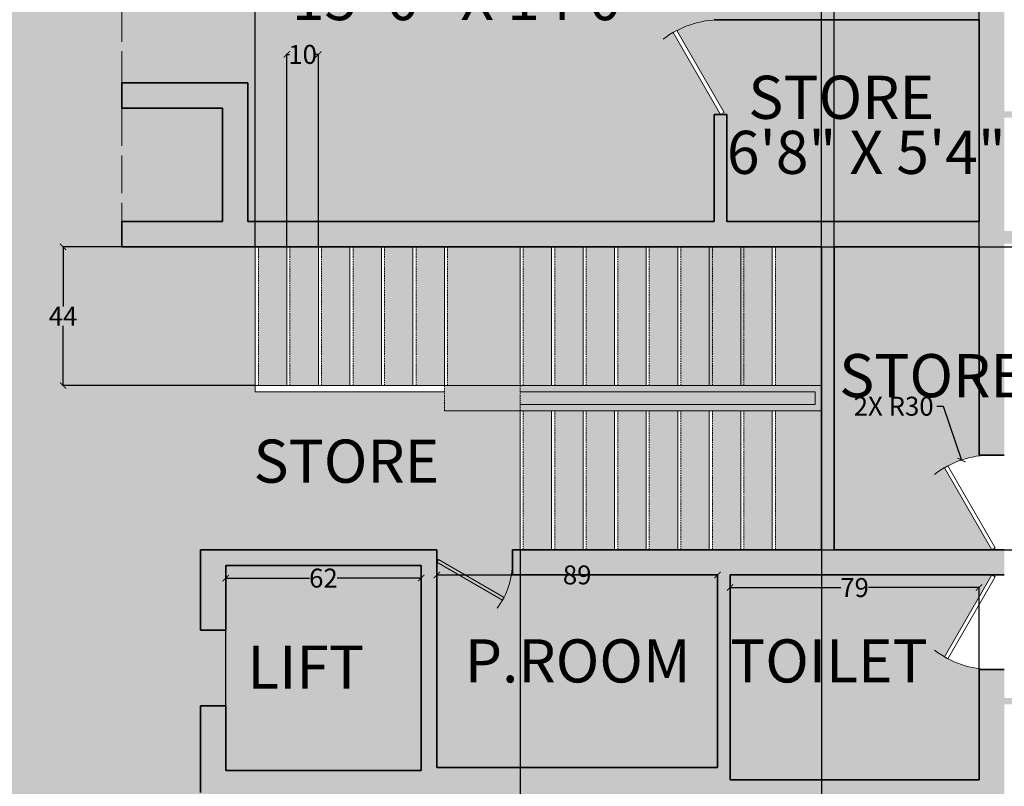
# Model space of a CAD drawing. Units: inches. Extents: x 1704 to 6393, y -157 to 1172.
# Tile 87 of 122: x 2293 to 2605, y 540 to 783. Entities that reach past the tile are written whole.
import ezdxf

# ---------------------------------------------------------------- set-up
doc = ezdxf.new("R2010")
doc.units = ezdxf.units.IN
doc.header["$MEASUREMENT"] = 0
doc.linetypes.add('ACAD_ISO02W100', pattern=[15, 12, -3])
doc.linetypes.add('DASHED', pattern=[0.75, 0.5, -0.25])
for name, color, linetype, lineweight in [('A-ANNO-DIMS', 7, 'Continuous', 13), ('A-AREA-IDEN', 7, 'Continuous', 18), ('A-FLOR-STRS-HIDN', 8, 'DASHED', 13), ('A-WALL-OVHD', 8, 'ACAD_ISO02W100', 13), ('A-WALL-PATT', 7, 'Continuous', 13), ('DOORS', 160, 'Continuous', 18), ('STAIRS', 7, 'Continuous', 18), ('WALLS', 7, 'Continuous', 35)]:
    doc.layers.add(name, color=color, linetype=linetype, lineweight=lineweight)
doc.layers.add('A-FLOR-PATT', color=7, linetype='Continuous', lineweight=13, true_color=0xf2f2f2)
doc.styles.get("Standard").update_dxf_attribs({"font": 'arial.ttf'})
doc.dimstyles.get("Standard").update_dxf_attribs({"dimtxt": 6, "dimasz": 2, "dimexe": 0.18, "dimexo": 0.0625, "dimgap": 0.09, "dimtad": 0, "dimtih": 1, "dimtoh": 1, "dimdec": 1, "dimzin": 0, "dimdsep": 46, "dimlunit": 3, "dimtxsty": 'Standard', "dimblk": 'ARCHTICK', "dimcen": 0.09, "dimadec": 0, "dimazin": 0, "dimtfac": 1, "dimtdec": 1, "dimtofl": 0, "dimtmove": 0, "dimatfit": 3, "dimfxl": 1, "dimtolj": 1, "dimtzin": 0, "dimarcsym": 0})

# ---------------------------------------------------------------- blocks, each defined once
blk = doc.blocks.new('Door - Left Hung 36 in.')
blk.add_lwpolyline([(0.75, -1.3), (0, 0), (31.18, 18), (31.93, 16.7)], close=True)
blk.add_arc((0, 0), 36, 0, 37.3101)
blk = doc.blocks.new('_ArchTick')
at = {"color": 0, "linetype": 'ByBlock', "const_width": 0.15}
blk.add_lwpolyline([(-0.5, -0.5), (0.5, 0.5)], dxfattribs=at)
blk = doc.blocks.new('*D93')
at = {"layer": 'A-ANNO-DIMS', "color": 0, "lineweight": -2, "transparency": 16777216}
for p, q in [((2605.29, 895.21), (1829.7, 895.21)), ((1829.88, 895.21), (1829.88, 495.87)), ((1829.88, 90.21), (1829.88, 489.56)), ((2605.29, 90.21), (1829.7, 90.21))]:
    blk.add_line(p, q, dxfattribs=at)
at = {"layer": 'Defpoints', "color": 0, "lineweight": -3, "transparency": 16777216}
for p in [(2605.35, 895.21), (1829.88, 90.21), (2605.35, 90.21)]:
    blk.add_point(p, dxfattribs=at)
at = {"layer": 'A-ANNO-DIMS', "color": 0, "lineweight": -2, "transparency": 16777216, "xscale": 2, "yscale": 2, "zscale": 2}
for p, rotation in [((1829.88, 895.21), 90), ((1829.88, 90.21), 270)]:
    blk.add_blockref('_ArchTick', p, dxfattribs=dict(at, rotation=rotation))
at = {"layer": 'A-ANNO-DIMS', "color": 0, "transparency": 16777216, "insert": (1829.88, 492.71), "char_height": 6, "attachment_point": 5}
blk.add_mtext('\\A1;805', dxfattribs=at)
blk = doc.blocks.new('*D98')
at = {"layer": 'A-ANNO-DIMS', "color": 0, "lineweight": -2, "transparency": 16777216}
for p, q in [((2358.35, 545.28), (2358.35, 606.39)), ((2358.35, 606.21), (2384.98, 606.21)), ((2420.35, 606.21), (2393.72, 606.21)), ((2420.35, 545.28), (2420.35, 606.39))]:
    blk.add_line(p, q, dxfattribs=at)
at = {"layer": 'Defpoints', "color": 0, "lineweight": -3, "transparency": 16777216}
for p in [(2420.35, 606.21), (2358.35, 545.21), (2420.35, 545.21)]:
    blk.add_point(p, dxfattribs=at)
at = {"layer": 'A-ANNO-DIMS', "color": 0, "lineweight": -2, "transparency": 16777216, "xscale": 2, "yscale": 2, "zscale": 2, "rotation": 180}
blk.add_blockref('_ArchTick', (2358.35, 606.21), dxfattribs=at)
at = {"layer": 'A-ANNO-DIMS', "color": 0, "lineweight": -2, "transparency": 16777216, "xscale": 2, "yscale": 2, "zscale": 2}
blk.add_blockref('_ArchTick', (2420.35, 606.21), dxfattribs=at)
at = {"layer": 'A-ANNO-DIMS', "color": 0, "transparency": 16777216, "insert": (2389.35, 606.21), "char_height": 6, "attachment_point": 5}
blk.add_mtext('\\A1;62', dxfattribs=at)
blk = doc.blocks.new('*D99')
at = {"layer": 'A-ANNO-DIMS', "color": 0, "lineweight": -2, "transparency": 16777216}
for p, q in [((2425.35, 546.28), (2425.35, 607.39)), ((2425.35, 607.21), (2465.45, 607.21)), ((2514.35, 607.21), (2474.25, 607.21)), ((2514.35, 546.28), (2514.35, 607.39))]:
    blk.add_line(p, q, dxfattribs=at)
at = {"layer": 'Defpoints', "color": 0, "lineweight": -3, "transparency": 16777216}
for p in [(2514.35, 607.21), (2425.35, 546.21), (2514.35, 546.21)]:
    blk.add_point(p, dxfattribs=at)
at = {"layer": 'A-ANNO-DIMS', "color": 0, "lineweight": -2, "transparency": 16777216, "xscale": 2, "yscale": 2, "zscale": 2, "rotation": 180}
blk.add_blockref('_ArchTick', (2425.35, 607.21), dxfattribs=at)
at = {"layer": 'A-ANNO-DIMS', "color": 0, "lineweight": -2, "transparency": 16777216, "xscale": 2, "yscale": 2, "zscale": 2}
blk.add_blockref('_ArchTick', (2514.35, 607.21), dxfattribs=at)
at = {"layer": 'A-ANNO-DIMS', "color": 0, "transparency": 16777216, "insert": (2469.85, 607.21), "char_height": 6, "attachment_point": 5}
blk.add_mtext('\\A1;89', dxfattribs=at)
blk = doc.blocks.new('*D100')
at = {"layer": 'A-ANNO-DIMS', "color": 0, "lineweight": -2, "transparency": 16777216}
for p, q in [((2518.35, 542.28), (2518.35, 603.39)), ((2518.35, 603.21), (2553.48, 603.21)), ((2597.35, 603.21), (2562.22, 603.21)), ((2597.35, 542.28), (2597.35, 603.39))]:
    blk.add_line(p, q, dxfattribs=at)
at = {"layer": 'Defpoints', "color": 0, "lineweight": -3, "transparency": 16777216}
for p in [(2597.35, 603.21), (2518.35, 542.21), (2597.35, 542.21)]:
    blk.add_point(p, dxfattribs=at)
at = {"layer": 'A-ANNO-DIMS', "color": 0, "lineweight": -2, "transparency": 16777216, "xscale": 2, "yscale": 2, "zscale": 2, "rotation": 180}
blk.add_blockref('_ArchTick', (2518.35, 603.21), dxfattribs=at)
at = {"layer": 'A-ANNO-DIMS', "color": 0, "lineweight": -2, "transparency": 16777216, "xscale": 2, "yscale": 2, "zscale": 2}
blk.add_blockref('_ArchTick', (2597.35, 603.21), dxfattribs=at)
at = {"layer": 'A-ANNO-DIMS', "color": 0, "transparency": 16777216, "insert": (2557.85, 603.21), "char_height": 6, "attachment_point": 5}
blk.add_mtext('\\A1;79', dxfattribs=at)
blk = doc.blocks.new('*D101')
at = {"layer": 'A-ANNO-DIMS', "color": 0, "lineweight": -2, "transparency": 16777216}
for p, q in [((2547.41, 711.21), (2784.53, 711.21)), ((2784.35, 711.21), (2784.35, 666.37)), ((2784.35, 615.21), (2784.35, 660.06)), ((2547.41, 615.21), (2784.53, 615.21))]:
    blk.add_line(p, q, dxfattribs=at)
at = {"layer": 'Defpoints', "color": 0, "lineweight": -3, "transparency": 16777216}
for p in [(2547.35, 711.21), (2784.35, 711.21), (2547.35, 615.21)]:
    blk.add_point(p, dxfattribs=at)
at = {"layer": 'A-ANNO-DIMS', "color": 0, "lineweight": -2, "transparency": 16777216, "xscale": 2, "yscale": 2, "zscale": 2}
for p, rotation in [((2784.35, 711.21), 90), ((2784.35, 615.21), 270)]:
    blk.add_blockref('_ArchTick', p, dxfattribs=dict(at, rotation=rotation))
at = {"layer": 'A-ANNO-DIMS', "color": 0, "transparency": 16777216, "insert": (2784.35, 663.21), "char_height": 6, "attachment_point": 5}
blk.add_mtext('\\A1;96', dxfattribs=at)
blk = doc.blocks.new('*D102')
at = {"layer": 'A-ANNO-DIMS', "color": 0, "lineweight": -2, "transparency": 16777216}
for p, q in [((2367.74, 711.28), (2367.74, 1105.29)), ((2367.74, 1105.11), (2447.61, 1105.11)), ((2547.35, 1105.11), (2467.47, 1105.11)), ((2547.35, 711.28), (2547.35, 1105.29))]:
    blk.add_line(p, q, dxfattribs=at)
at = {"layer": 'Defpoints', "color": 0, "lineweight": -3, "transparency": 16777216}
for p in [(2547.35, 1105.11), (2367.74, 711.21), (2547.35, 711.21)]:
    blk.add_point(p, dxfattribs=at)
at = {"layer": 'A-ANNO-DIMS', "color": 0, "lineweight": -2, "transparency": 16777216, "xscale": 2, "yscale": 2, "zscale": 2, "rotation": 180}
blk.add_blockref('_ArchTick', (2367.74, 1105.11), dxfattribs=at)
at = {"layer": 'A-ANNO-DIMS', "color": 0, "lineweight": -2, "transparency": 16777216, "xscale": 2, "yscale": 2, "zscale": 2}
blk.add_blockref('_ArchTick', (2547.35, 1105.11), dxfattribs=at)
at = {"layer": 'A-ANNO-DIMS', "color": 0, "transparency": 16777216, "insert": (2457.54, 1105.11), "char_height": 6, "attachment_point": 5}
blk.add_mtext('\\A1;179.6', dxfattribs=at)
blk = doc.blocks.new('*D103')
at = {"layer": 'A-ANNO-DIMS', "color": 0, "lineweight": -2, "transparency": 16777216}
for p, q in [((2551.35, 711.28), (2551.35, 1105.29)), ((2551.35, 1105.11), (2569.84, 1105.11)), ((2597.35, 1105.11), (2578.85, 1105.11)), ((2597.35, 711.28), (2597.35, 1105.29))]:
    blk.add_line(p, q, dxfattribs=at)
at = {"layer": 'Defpoints', "color": 0, "lineweight": -3, "transparency": 16777216}
for p in [(2597.35, 1105.11), (2551.35, 711.21), (2597.35, 711.21)]:
    blk.add_point(p, dxfattribs=at)
at = {"layer": 'A-ANNO-DIMS', "color": 0, "lineweight": -2, "transparency": 16777216, "xscale": 2, "yscale": 2, "zscale": 2, "rotation": 180}
blk.add_blockref('_ArchTick', (2551.35, 1105.11), dxfattribs=at)
at = {"layer": 'A-ANNO-DIMS', "color": 0, "lineweight": -2, "transparency": 16777216, "xscale": 2, "yscale": 2, "zscale": 2}
blk.add_blockref('_ArchTick', (2597.35, 1105.11), dxfattribs=at)
at = {"layer": 'A-ANNO-DIMS', "color": 0, "transparency": 16777216, "insert": (2574.35, 1105.11), "char_height": 6, "attachment_point": 5}
blk.add_mtext('\\A1;46', dxfattribs=at)
blk = doc.blocks.new('*D104')
at = {"layer": 'A-ANNO-DIMS', "color": 0, "lineweight": -2, "transparency": 16777216}
for p, q in [((2367.675475, 711.212974), (2306.557975, 711.212974)), ((2306.737975, 711.212974), (2306.737975, 692.302974)), ((2306.737975, 667.212974), (2306.737975, 686.122974)), ((2367.675475, 667.212974), (2306.557975, 667.212974))]:
    blk.add_line(p, q, dxfattribs=at)
at = {"layer": 'Defpoints', "color": 0, "lineweight": -3, "transparency": 16777216}
for p in [(2306.737975, 711.212974), (2367.737975, 711.212974), (2367.737975, 667.212974)]:
    blk.add_point(p, dxfattribs=at)
at = {"layer": 'A-ANNO-DIMS', "color": 0, "lineweight": -2, "transparency": 16777216, "xscale": 2, "yscale": 2, "zscale": 2}
for p, rotation in [((2306.737975, 711.212974), 90), ((2306.737975, 667.212974), 270)]:
    blk.add_blockref('_ArchTick', p, dxfattribs=dict(at, rotation=rotation))
at = {"layer": 'A-ANNO-DIMS', "color": 0, "transparency": 16777216, "insert": (2306.737975, 689.212974), "char_height": 6, "attachment_point": 5}
blk.add_mtext('\\A1;44', dxfattribs=at)
blk = doc.blocks.new('*D105')
at = {"layer": 'A-ANNO-DIMS', "color": 0, "lineweight": -2, "transparency": 16777216}
for p, q in [((2451.74, 615.15), (2451.74, -64.97)), ((2547.35, 615.15), (2547.35, -64.97)), ((2451.74, -64.79), (2489.91, -64.79)), ((2547.35, -64.79), (2509.18, -64.79))]:
    blk.add_line(p, q, dxfattribs=at)
at = {"layer": 'Defpoints', "color": 0, "lineweight": -3, "transparency": 16777216}
for p in [(2451.74, 615.21), (2547.35, 615.21), (2547.35, -64.79)]:
    blk.add_point(p, dxfattribs=at)
at = {"layer": 'A-ANNO-DIMS', "color": 0, "lineweight": -2, "transparency": 16777216, "xscale": 2, "yscale": 2, "zscale": 2, "rotation": 180}
blk.add_blockref('_ArchTick', (2451.74, -64.79), dxfattribs=at)
at = {"layer": 'A-ANNO-DIMS', "color": 0, "lineweight": -2, "transparency": 16777216, "xscale": 2, "yscale": 2, "zscale": 2}
blk.add_blockref('_ArchTick', (2547.35, -64.79), dxfattribs=at)
at = {"layer": 'A-ANNO-DIMS', "color": 0, "transparency": 16777216, "insert": (2499.54, -64.79), "char_height": 6, "attachment_point": 5}
blk.add_mtext('\\A1;95.61', dxfattribs=at)
blk = doc.blocks.new('*D106')
at = {"layer": 'A-ANNO-DIMS', "color": 0, "lineweight": -2, "transparency": 16777216}
for p, q in [((2377.74, 711.28), (2377.74, 772.39)), ((2377.74, 772.21), (2378.64, 772.21)), ((2387.74, 772.21), (2386.83, 772.21)), ((2387.74, 711.28), (2387.74, 772.39))]:
    blk.add_line(p, q, dxfattribs=at)
at = {"layer": 'Defpoints', "color": 0, "lineweight": -3, "transparency": 16777216}
for p in [(2387.74, 772.21), (2377.74, 711.21), (2387.74, 711.21)]:
    blk.add_point(p, dxfattribs=at)
at = {"layer": 'A-ANNO-DIMS', "color": 0, "lineweight": -2, "transparency": 16777216, "xscale": 2, "yscale": 2, "zscale": 2, "rotation": 180}
blk.add_blockref('_ArchTick', (2377.74, 772.21), dxfattribs=at)
at = {"layer": 'A-ANNO-DIMS', "color": 0, "lineweight": -2, "transparency": 16777216, "xscale": 2, "yscale": 2, "zscale": 2}
blk.add_blockref('_ArchTick', (2387.74, 772.21), dxfattribs=at)
at = {"layer": 'A-ANNO-DIMS', "color": 0, "transparency": 16777216, "insert": (2382.74, 772.21), "char_height": 6, "attachment_point": 5}
blk.add_mtext('\\A1;10', dxfattribs=at)
blk = doc.blocks.new('*D136')
at = {"layer": 'A-ANNO-DIMS', "color": 0, "lineweight": -2, "transparency": 16777216}
for p, q in [((2583.99, 660.69), (2585.99, 660.69)), ((2585.99, 660.69), (2591.75, 643.64)), ((2601.26, 615.21), (2601.44, 615.21)), ((2601.35, 615.12), (2601.35, 615.3))]:
    blk.add_line(p, q, dxfattribs=at)
at = {"layer": 'Defpoints', "color": 0, "lineweight": -3, "transparency": 16777216}
for p in [(2591.75, 643.64), (2601.35, 615.21)]:
    blk.add_point(p, dxfattribs=at)
at = {"layer": 'A-ANNO-DIMS', "color": 0, "lineweight": -2, "transparency": 16777216, "xscale": 2, "yscale": 2, "zscale": 2, "rotation": 288.6558092549602}
blk.add_blockref('_ArchTick', (2591.75, 643.64), dxfattribs=at)
at = {"layer": 'A-ANNO-DIMS', "color": 0, "transparency": 16777216, "insert": (2570.25, 660.69), "char_height": 6, "attachment_point": 5}
blk.add_mtext('\\A1;2X R30', dxfattribs=at)

msp = doc.modelspace()

# ---------------------------------------------------------------- hatches: boundary and pattern name
at = {"layer": 'A-FLOR-PATT', "transparency": 33554528}
h = msp.add_hatch(color=256, dxfattribs=at)
h.dxf.hatch_style = 1
h.paths.add_polyline_path([(2325.349, 863.213), (2325.349, 887.213), (2263.349, 887.213), (2167.349, 887.213), (2081.349, 887.213), (2081.349, 719.213), (2277.349, 719.213), (2277.349, 711.213), (2277.349, 372.213), (2349.349, 372.213), (2381.349, 372.213), (2381.349, 364.213), (2353.349, 364.213), (2353.349, 270.213), (2381.349, 270.213), (2381.349, 266.213), (2357.349, 266.213), (2357.349, 98.213), (2381.349, 98.213), (2385.181, 98.213), (2386.482, 98.213), (2424.215, 98.213), (2425.516, 98.213), (2429.349, 98.213), (2597.349, 98.213), (2597.349, 146.213), (2597.349, 218.213), (2597.349, 266.213), (2423.349, 266.213), (2423.349, 270.213), (2473.349, 270.213), (2473.349, 294.213), (2477.349, 294.213), (2477.349, 270.213), (2547.349, 270.213), (2547.349, 364.213), (2477.349, 364.213), (2477.349, 318.213), (2473.349, 318.213), (2473.349, 364.213), (2423.349, 364.213), (2423.349, 372.213), (2469.349, 372.213), (2469.349, 459.213), (2469.349, 538.213), (2350.349, 538.213), (2350.349, 565.713), (2358.349, 565.713), (2358.349, 545.213), (2420.349, 545.213), (2420.349, 610.213), (2358.349, 610.213), (2358.349, 589.713), (2350.349, 589.713), (2350.349, 615.213), (2425.349, 615.213), (2425.349, 607.213), (2425.349, 546.213), (2469.349, 546.213), (2514.349, 546.213), (2514.349, 607.213), (2449.349, 607.213), (2449.349, 615.213), (2451.738, 615.213), (2451.738, 659.213), (2427.738, 659.213), (2427.738, 665.213), (2367.738, 665.213), (2367.738, 667.213), (2367.738, 711.213), (2325.349, 711.213), (2325.349, 719.213), (2325.349, 755.213), (2325.349, 763.213)])
h.paths.add_polyline_path([(2233.858, 822.533, -0.187247), (2233.858, 809.14), (2231.697, 808.804, 0.0848928), (2233.131, 814.486), (2230.424, 814.486, -0.1042581), (2228.553, 808.313), (2217.751, 807.156, -0.2222222), (2217.751, 824.517), (2228.553, 823.359, -0.1042581), (2230.424, 817.186), (2233.131, 817.186, 0.0848928), (2231.697, 822.868)], flags=16)
h.paths.add_polyline_path([(2213.621, 833.197), (2213.621, 798.475), (2156.048, 798.475), (2156.048, 833.197)], flags=16)
h.paths.add_polyline_path([(2203.932, 848.099), (2205.089, 837.296, -0.2222222), (2187.728, 837.296), (2188.885, 848.099, -0.1042581), (2195.058, 849.969), (2195.058, 852.676, 0.0848928), (2189.377, 851.242), (2189.712, 853.404, -0.187247), (2203.105, 853.404), (2203.44, 851.242, 0.0848928), (2197.759, 852.676), (2197.759, 849.969, -0.1042581)], flags=16)
h.paths.add_polyline_path([(2181.941, 837.296, -0.2222222), (2164.58, 837.296), (2165.737, 848.099, -0.1042581), (2171.91, 849.969), (2171.91, 852.676, 0.0848928), (2166.229, 851.242), (2166.564, 853.404, -0.187247), (2179.957, 853.404), (2180.292, 851.242, 0.0848928), (2174.611, 852.676), (2174.611, 849.969, -0.1042581), (2180.784, 848.099)], flags=16)
h.paths.add_polyline_path([(2205.089, 794.376), (2203.932, 783.574, -0.1042581), (2197.759, 781.703), (2197.759, 778.996, 0.0848928), (2203.44, 780.43), (2203.105, 778.269, -0.187247), (2189.712, 778.269), (2189.377, 780.43, 0.0848928), (2195.058, 778.996), (2195.058, 781.703, -0.1042581), (2188.885, 783.574), (2187.728, 794.376, -0.2222222)], flags=16)
h.paths.add_polyline_path([(2181.941, 794.376), (2180.784, 783.574, -0.1042581), (2174.611, 781.703), (2174.611, 778.996, 0.0848928), (2180.292, 780.43), (2179.957, 778.269, -0.187247), (2166.564, 778.269), (2166.229, 780.43, 0.0848928), (2171.91, 778.996), (2171.91, 781.703, -0.1042581), (2165.737, 783.574), (2164.58, 794.376, -0.2222222)], flags=16)
h.paths.add_polyline_path([(2151.918, 807.156), (2141.116, 808.313, -0.1042581), (2139.245, 814.486), (2136.539, 814.486, 0.0848928), (2137.972, 808.804), (2135.811, 809.14, -0.187247), (2135.811, 822.533), (2137.972, 822.868, 0.0848928), (2136.539, 817.186), (2139.245, 817.186, -0.1042581), (2141.116, 823.359), (2151.918, 824.517, -0.2222222)], flags=16)
h.paths.add_polyline_path([(2357.868, 363.41), (2358.814, 363.41, 0.7537605)], flags=16)
h.paths.add_polyline_path([(2372.241, 363.117), (2372.248, 363.117), (2372.248, 363.343), (2371.302, 363.343), (2371.302, 363.139, -1.3603913)], flags=16)
h.paths.add_polyline_path([(2371.309, 272.716), (2371.302, 272.716), (2371.302, 272.49), (2372.248, 272.49), (2372.248, 272.693, -1.3603913)], flags=16)
h.paths.add_polyline_path([(2357.875, 272.716), (2357.868, 272.716), (2357.868, 272.49), (2358.814, 272.49), (2358.814, 272.693, -1.3603913)], flags=16)
h.paths.add_polyline_path([(2353.769, 363.074), (2376.347, 363.074), (2376.347, 272.759), (2353.769, 272.759)], flags=16)
h.paths.add_polyline_path([(2354.772, 362.07), (2375.344, 362.07), (2375.344, 273.762), (2354.772, 273.762)], flags=0)
h.paths.add_polyline_path([(2357.868, 363.343), (2358.814, 363.343), (2358.814, 363.117), (2357.868, 363.117)], flags=16)
h.paths.add_polyline_path([(2359.288, 359.184), (2359.288, 360.063), (2370.828, 360.063), (2370.828, 359.184), (2374.332, 359.184), (2374.332, 358.464), (2372.835, 358.464), (2372.835, 357.541), (2374.332, 357.541), (2374.332, 356.82), (2372.835, 356.82), (2372.835, 355.898), (2374.332, 355.898), (2374.332, 355.177), (2372.835, 355.177), (2372.835, 354.254), (2374.332, 354.254), (2374.332, 353.534), (2372.835, 353.534), (2372.835, 352.611), (2374.332, 352.611), (2374.332, 351.89), (2372.835, 351.89), (2372.835, 350.968), (2374.332, 350.968), (2374.332, 350.247), (2372.835, 350.247), (2372.835, 349.324), (2374.332, 349.324), (2374.332, 348.604), (2372.835, 348.604), (2372.835, 347.681), (2374.332, 347.681), (2374.332, 346.96), (2372.835, 346.96), (2372.835, 346.038), (2374.332, 346.038), (2374.332, 345.317), (2372.835, 345.317), (2372.835, 344.395), (2374.332, 344.395), (2374.332, 343.674), (2372.835, 343.674), (2372.835, 342.751), (2374.332, 342.751), (2374.332, 342.03), (2372.835, 342.03), (2372.835, 341.108), (2374.332, 341.108), (2374.332, 340.387), (2372.835, 340.387), (2372.835, 339.465), (2374.332, 339.465), (2374.332, 338.744), (2372.835, 338.744), (2372.835, 337.821), (2374.332, 337.821), (2374.332, 337.1), (2372.835, 337.1), (2372.835, 336.178), (2374.332, 336.178), (2374.332, 335.457), (2372.835, 335.457), (2372.835, 334.535), (2374.332, 334.535), (2374.332, 333.814), (2372.835, 333.814), (2372.835, 332.891), (2374.332, 332.891), (2374.332, 332.171), (2372.835, 332.171), (2372.835, 331.248), (2374.332, 331.248), (2374.332, 330.527), (2372.835, 330.527), (2372.835, 329.605), (2374.332, 329.605), (2374.332, 328.884), (2372.835, 328.884), (2372.835, 327.961), (2374.332, 327.961), (2374.332, 327.241), (2372.835, 327.241), (2372.835, 326.318), (2374.332, 326.318), (2374.332, 325.597), (2372.835, 325.597), (2372.835, 324.675), (2374.332, 324.675), (2374.332, 323.954), (2372.835, 323.954), (2372.835, 323.031), (2374.332, 323.031), (2374.332, 322.311), (2372.835, 322.311), (2372.835, 321.388), (2374.332, 321.388), (2374.332, 320.667), (2372.835, 320.667), (2372.835, 319.745), (2374.332, 319.745), (2374.332, 319.024), (2372.835, 319.024), (2372.835, 318.102), (2374.332, 318.102), (2374.332, 317.381), (2372.835, 317.381), (2372.835, 316.458), (2374.332, 316.458), (2374.332, 315.737), (2372.835, 315.737), (2372.835, 314.815), (2374.332, 314.815), (2374.332, 314.094), (2372.835, 314.094), (2372.835, 313.172), (2374.332, 313.172), (2374.332, 312.451), (2372.835, 312.451), (2372.835, 311.528), (2374.332, 311.528), (2374.332, 310.807), (2372.835, 310.807), (2372.835, 309.885), (2374.332, 309.885), (2374.332, 309.164), (2372.835, 309.164), (2372.835, 308.242), (2374.332, 308.242), (2374.332, 307.521), (2372.835, 307.521), (2372.835, 306.598), (2374.332, 306.598), (2374.332, 305.878), (2372.835, 305.878), (2372.835, 304.955), (2374.332, 304.955), (2374.332, 304.234), (2372.835, 304.234), (2372.835, 303.312), (2374.332, 303.312), (2374.332, 302.591), (2372.835, 302.591), (2372.835, 301.668), (2374.332, 301.668), (2374.332, 300.948), (2372.835, 300.948), (2372.835, 300.025), (2374.332, 300.025), (2374.332, 299.304), (2372.835, 299.304), (2372.835, 298.382), (2374.332, 298.382), (2374.332, 297.661), (2372.835, 297.661), (2372.835, 296.738), (2374.332, 296.738), (2374.332, 296.018), (2372.835, 296.018), (2372.835, 295.095), (2374.332, 295.095), (2374.332, 294.374), (2372.835, 294.374), (2372.835, 293.452), (2374.332, 293.452), (2374.332, 292.731), (2372.835, 292.731), (2372.835, 291.809), (2374.332, 291.809), (2374.332, 291.088), (2372.835, 291.088), (2372.835, 290.165), (2374.332, 290.165), (2374.332, 289.444), (2372.835, 289.444), (2372.835, 288.522), (2374.332, 288.522), (2374.332, 287.801), (2372.835, 287.801), (2372.835, 286.879), (2374.332, 286.879), (2374.332, 286.158), (2372.835, 286.158), (2372.835, 285.235), (2374.332, 285.235), (2374.332, 284.514), (2372.835, 284.514), (2372.835, 283.592), (2374.332, 283.592), (2374.332, 282.871), (2372.835, 282.871), (2372.835, 281.949), (2374.332, 281.949), (2374.332, 281.228), (2372.835, 281.228), (2372.835, 280.305), (2374.332, 280.305), (2374.332, 279.585), (2372.835, 279.585), (2372.835, 278.662), (2374.332, 278.662), (2374.332, 277.941), (2372.835, 277.941), (2372.835, 277.019), (2374.332, 277.019), (2374.332, 276.298), (2370.828, 276.298), (2370.828, 275.769), (2359.288, 275.769), (2359.288, 276.298), (2355.784, 276.298), (2355.784, 277.019), (2357.281, 277.019), (2357.281, 277.941), (2355.784, 277.941), (2355.784, 278.662), (2357.281, 278.662), (2357.281, 279.585), (2355.784, 279.585), (2355.784, 280.305), (2357.281, 280.305), (2357.281, 281.228), (2355.784, 281.228), (2355.784, 281.949), (2357.281, 281.949), (2357.281, 282.871), (2355.784, 282.871), (2355.784, 283.592), (2357.281, 283.592), (2357.281, 284.514), (2355.784, 284.514), (2355.784, 285.235), (2357.281, 285.235), (2357.281, 286.158), (2355.784, 286.158), (2355.784, 286.879), (2357.281, 286.879), (2357.281, 287.801), (2355.784, 287.801), (2355.784, 288.522), (2357.281, 288.522), (2357.281, 289.444), (2355.784, 289.444), (2355.784, 290.165), (2357.281, 290.165), (2357.281, 291.088), (2355.784, 291.088), (2355.784, 291.809), (2357.281, 291.809), (2357.281, 292.731), (2355.784, 292.731), (2355.784, 293.452), (2357.281, 293.452), (2357.281, 294.374), (2355.784, 294.374), (2355.784, 295.095), (2357.281, 295.095), (2357.281, 296.018), (2355.784, 296.018), (2355.784, 296.738), (2357.281, 296.738), (2357.281, 297.661), (2355.784, 297.661), (2355.784, 298.382), (2357.281, 298.382), (2357.281, 299.304), (2355.784, 299.304), (2355.784, 300.025), (2357.281, 300.025), (2357.281, 300.948), (2355.784, 300.948), (2355.784, 301.668), (2357.281, 301.668), (2357.281, 302.591), (2355.784, 302.591), (2355.784, 303.312), (2357.281, 303.312), (2357.281, 304.234), (2355.784, 304.234), (2355.784, 304.955), (2357.281, 304.955), (2357.281, 305.878), (2355.784, 305.878), (2355.784, 306.598), (2357.281, 306.598), (2357.281, 307.521), (2355.784, 307.521), (2355.784, 308.242), (2357.281, 308.242), (2357.281, 309.164), (2355.784, 309.164), (2355.784, 309.885), (2357.281, 309.885), (2357.281, 310.807), (2355.784, 310.807), (2355.784, 311.528), (2357.281, 311.528), (2357.281, 312.451), (2355.784, 312.451), (2355.784, 313.172), (2357.281, 313.172), (2357.281, 314.094), (2355.784, 314.094), (2355.784, 314.815), (2357.281, 314.815), (2357.281, 315.737), (2355.784, 315.737), (2355.784, 316.458), (2357.281, 316.458), (2357.281, 317.381), (2355.784, 317.381), (2355.784, 318.102), (2357.281, 318.102), (2357.281, 319.024), (2355.784, 319.024), (2355.784, 319.745), (2357.281, 319.745), (2357.281, 320.667), (2355.784, 320.667), (2355.784, 321.388), (2357.281, 321.388), (2357.281, 322.311), (2355.784, 322.311), (2355.784, 323.031), (2357.281, 323.031), (2357.281, 323.954), (2355.784, 323.954), (2355.784, 324.675), (2357.281, 324.675), (2357.281, 325.597), (2355.784, 325.597), (2355.784, 326.318), (2357.281, 326.318), (2357.281, 327.241), (2355.784, 327.241), (2355.784, 327.961), (2357.281, 327.961), (2357.281, 328.884), (2355.784, 328.884), (2355.784, 329.605), (2357.281, 329.605), (2357.281, 330.527), (2355.784, 330.527), (2355.784, 331.248), (2357.281, 331.248), (2357.281, 332.171), (2355.784, 332.171), (2355.784, 332.891), (2357.281, 332.891), (2357.281, 333.814), (2355.784, 333.814), (2355.784, 334.535), (2357.281, 334.535), (2357.281, 335.457), (2355.784, 335.457), (2355.784, 336.178), (2357.281, 336.178), (2357.281, 337.1), (2355.784, 337.1), (2355.784, 337.821), (2357.281, 337.821), (2357.281, 338.744), (2355.784, 338.744), (2355.784, 339.465), (2357.281, 339.465), (2357.281, 340.387), (2355.784, 340.387), (2355.784, 341.108), (2357.281, 341.108), (2357.281, 342.03), (2355.784, 342.03), (2355.784, 342.751), (2357.281, 342.751), (2357.281, 343.674), (2355.784, 343.674), (2355.784, 344.395), (2357.281, 344.395), (2357.281, 345.317), (2355.784, 345.317), (2355.784, 346.038), (2357.281, 346.038), (2357.281, 346.96), (2355.784, 346.96), (2355.784, 347.681), (2357.281, 347.681), (2357.281, 348.604), (2355.784, 348.604), (2355.784, 349.324), (2357.281, 349.324), (2357.281, 350.247), (2355.784, 350.247), (2355.784, 350.968), (2357.281, 350.968), (2357.281, 351.89), (2355.784, 351.89), (2355.784, 352.611), (2357.281, 352.611), (2357.281, 353.534), (2355.784, 353.534), (2355.784, 354.254), (2357.281, 354.254), (2357.281, 355.177), (2355.784, 355.177), (2355.784, 355.898), (2357.281, 355.898), (2357.281, 356.82), (2355.784, 356.82), (2355.784, 357.541), (2357.281, 357.541), (2357.281, 358.464), (2355.784, 358.464), (2355.784, 359.184)], flags=0)
h = msp.add_hatch(color=256, dxfattribs=at)
h.dxf.hatch_style = 1
h.paths.add_polyline_path([(2517.349, 861.213), (2513.349, 861.213), (2513.349, 887.213), (2509.516, 887.213), (2508.215, 887.213), (2470.482, 887.213), (2469.181, 887.213), (2465.349, 887.213), (2333.349, 887.213), (2333.349, 863.213), (2325.349, 863.213), (2325.349, 763.213), (2365.349, 763.213), (2365.349, 719.213), (2513.349, 719.213), (2513.349, 753.213), (2515.349, 753.213), (2500.349, 779.194), (2501.431, 779.819), (2501.444, 779.796, -0.1041754), (2513.349, 783.146), (2513.349, 813.213), (2517.349, 813.213)])
h.paths.add_polyline_path([(2597.349, 818.213), (2601.349, 818.213), (2600.05, 818.963), (2618.034, 850.113, 0.1210664), (2601.349, 854.213), (2597.349, 854.213), (2597.349, 887.213), (2581.349, 887.213), (2533.349, 887.213), (2517.349, 887.213), (2517.349, 861.213), (2517.349, 813.213), (2517.349, 787.213), (2597.349, 787.213)])
h.paths.add_polyline_path([(2597.349, 783.213), (2517.349, 783.213), (2515.349, 783.213, 0.1210664), (2501.444, 779.796), (2516.792, 753.213), (2517.349, 753.213), (2517.349, 719.213), (2597.349, 719.213)])
h = msp.add_hatch(color=256, dxfattribs=at)
h.dxf.hatch_style = 1
h.paths.add_polyline_path([(2601.349, 451.213), (2597.349, 451.213), (2477.349, 451.213), (2477.349, 372.213), (2597.349, 372.213), (2597.349, 415.436, -0.0929107), (2584.663, 419.313), (2584.648, 419.286), (2583.349, 420.036)])
h.paths.add_polyline_path([(2583.349, 490.39), (2584.648, 491.14), (2584.663, 491.113, -0.0929107), (2597.349, 494.99), (2597.349, 538.213), (2477.349, 538.213), (2477.349, 459.213), (2597.349, 459.213), (2601.349, 459.213)])
h.paths.add_polyline_path([(2587.444, 580.63), (2587.431, 580.607), (2586.349, 581.232), (2601.349, 607.213), (2532.349, 607.213), (2518.349, 607.213), (2518.349, 542.213), (2597.349, 542.213), (2597.349, 577.481, -0.0872676)])
h.paths.add_polyline_path([(2597.349, 711.213), (2551.349, 711.213), (2551.349, 615.213), (2597.349, 615.213), (2601.349, 615.213), (2586.349, 641.194), (2587.431, 641.819), (2587.444, 641.796, -0.1210664), (2601.349, 645.213), (2597.349, 645.213)])
h.paths.add_polyline_path([(2547.349, 659.213), (2532.738, 659.213), (2532.738, 615.213), (2547.349, 615.213)])
h.paths.add_polyline_path([(2547.349, 711.213), (2532.738, 711.213), (2532.738, 667.213), (2547.349, 667.213)])
h.paths.add_polyline_path([(2357.349, 755.213), (2325.349, 755.213), (2325.349, 719.213), (2357.349, 719.213)])
h.paths.add_polyline_path([(2451.738, 711.213), (2428.738, 711.213), (2428.738, 667.213), (2451.738, 667.213)])
h.paths.add_polyline_path([(2427.738, 711.213), (2418.738, 711.213), (2418.738, 667.213), (2427.738, 667.213)])
h.paths.add_polyline_path([(2417.738, 711.213), (2408.738, 711.213), (2408.738, 667.213), (2417.738, 667.213)])
h.paths.add_polyline_path([(2407.738, 711.213), (2398.738, 711.213), (2398.738, 667.213), (2407.738, 667.213)])
h.paths.add_polyline_path([(2397.738, 711.213), (2388.738, 711.213), (2388.738, 667.213), (2397.738, 667.213)])
h.paths.add_polyline_path([(2387.738, 711.213), (2378.738, 711.213), (2378.738, 667.213), (2387.738, 667.213)])
h.paths.add_polyline_path([(2377.738, 711.213), (2368.738, 711.213), (2368.738, 667.213), (2377.738, 667.213)])
h.paths.add_polyline_path([(2461.738, 711.213), (2452.738, 711.213), (2452.738, 667.213), (2461.738, 667.213)])
h.paths.add_polyline_path([(2471.738, 711.213), (2462.738, 711.213), (2462.738, 667.213), (2471.738, 667.213)])
h.paths.add_polyline_path([(2481.738, 711.213), (2472.738, 711.213), (2472.738, 667.213), (2481.738, 667.213)])
h.paths.add_polyline_path([(2491.738, 711.213), (2482.738, 711.213), (2482.738, 667.213), (2491.738, 667.213)])
h.paths.add_polyline_path([(2501.738, 711.213), (2492.738, 711.213), (2492.738, 667.213), (2501.738, 667.213)])
h.paths.add_polyline_path([(2511.738, 711.213), (2502.738, 711.213), (2502.738, 667.213), (2511.738, 667.213)])
h.paths.add_polyline_path([(2521.738, 711.213), (2512.738, 711.213), (2512.738, 667.213), (2521.738, 667.213)])
h.paths.add_polyline_path([(2531.738, 711.213), (2522.738, 711.213), (2522.738, 667.213), (2531.738, 667.213)])
h.paths.add_polyline_path([(2522.738, 711.213), (2521.738, 711.213), (2521.738, 667.213), (2522.738, 667.213)])
h.paths.add_polyline_path([(2512.738, 711.213), (2511.738, 711.213), (2511.738, 667.213), (2512.738, 667.213)])
h.paths.add_polyline_path([(2531.738, 659.213), (2522.738, 659.213), (2522.738, 615.213), (2531.738, 615.213)])
h.paths.add_polyline_path([(2521.738, 659.213), (2512.738, 659.213), (2512.738, 615.213), (2521.738, 615.213)])
h.paths.add_polyline_path([(2511.738, 659.213), (2502.738, 659.213), (2502.738, 615.213), (2511.738, 615.213)])
h.paths.add_polyline_path([(2501.738, 659.213), (2492.738, 659.213), (2492.738, 615.213), (2501.738, 615.213)])
h.paths.add_polyline_path([(2491.738, 659.213), (2482.738, 659.213), (2482.738, 615.213), (2491.738, 615.213)])
h.paths.add_polyline_path([(2481.738, 659.213), (2472.738, 659.213), (2472.738, 615.213), (2481.738, 615.213)])
h.paths.add_polyline_path([(2471.738, 659.213), (2462.738, 659.213), (2462.738, 615.213), (2471.738, 615.213)])
h.paths.add_polyline_path([(2461.738, 659.213), (2452.738, 659.213), (2452.738, 615.213), (2461.738, 615.213)])
h.paths.add_polyline_path([(2545.349, 665.213), (2451.738, 665.213), (2451.738, 661.213), (2545.349, 661.213)], flags=17)
h.paths.add_polyline_path([(2547.349, 667.213), (2532.738, 667.213), (2451.738, 667.213), (2451.738, 665.213), (2545.349, 665.213), (2545.349, 661.213), (2451.738, 661.213), (2451.738, 659.213), (2547.349, 659.213)])
at = {"layer": 'A-WALL-PATT', "transparency": 33554643}
h = msp.add_hatch(color=256, dxfattribs=at)
h.dxf.hatch_style = 1
h.paths.add_polyline_path([(2167.349, 895.213), (2073.349, 895.213), (2073.349, 887.213), (2081.349, 887.213), (2167.349, 887.213)])
h.paths.add_polyline_path([(2465.349, 895.213), (2273.349, 895.213), (2273.349, 903.213), (2263.349, 903.213), (2263.349, 895.213), (2263.349, 887.213), (2325.349, 887.213), (2325.349, 863.213), (2333.349, 863.213), (2333.349, 887.213), (2465.349, 887.213)])
h.paths.add_polyline_path([(2533.349, 895.213), (2513.349, 895.213), (2513.349, 887.213), (2513.349, 861.213), (2517.349, 861.213), (2517.349, 887.213), (2533.349, 887.213)])
h.paths.add_polyline_path([(2605.349, 895.213), (2581.349, 895.213), (2581.349, 887.213), (2597.349, 887.213), (2597.349, 854.213), (2605.349, 854.213)])
h.paths.add_polyline_path([(2605.349, 752.213), (2629.349, 752.213), (2629.349, 716.213), (2605.349, 716.213), (2605.349, 712.213), (2719.349, 712.213), (2719.349, 716.213), (2631.349, 716.213), (2631.349, 754.213), (2605.349, 754.213), (2605.349, 794.213), (2597.349, 794.213), (2597.349, 787.213), (2517.349, 787.213), (2517.349, 813.213), (2513.349, 813.213), (2513.349, 783.213), (2517.349, 783.213), (2597.349, 783.213), (2597.349, 719.213), (2517.349, 719.213), (2517.349, 753.213), (2513.349, 753.213), (2513.349, 719.213), (2365.349, 719.213), (2365.349, 763.213), (2325.349, 763.213), (2325.349, 755.213), (2357.349, 755.213), (2357.349, 719.213), (2325.349, 719.213), (2325.349, 711.213), (2547.349, 711.213), (2547.349, 615.213), (2449.349, 615.213), (2449.349, 607.213), (2514.349, 607.213), (2514.349, 546.213), (2439.349, 546.213), (2425.349, 546.213), (2425.349, 607.213), (2425.349, 615.213), (2350.349, 615.213), (2350.349, 589.713), (2358.349, 589.713), (2358.349, 610.213), (2420.349, 610.213), (2420.349, 545.213), (2358.349, 545.213), (2358.349, 565.713), (2350.349, 565.713), (2350.349, 538.213), (2469.349, 538.213), (2469.349, 459.213), (2469.349, 372.213), (2423.349, 372.213), (2423.349, 364.213), (2473.349, 364.213), (2473.349, 318.213), (2477.349, 318.213), (2477.349, 364.213), (2547.349, 364.213), (2547.349, 352.213), (2549.349, 352.213), (2549.349, 364.213), (2597.349, 364.213), (2597.349, 328.213), (2549.349, 328.213), (2547.349, 328.213), (2547.349, 326.213), (2549.349, 326.213), (2597.349, 326.213), (2605.349, 326.213), (2605.349, 377.057), (2597.349, 377.057), (2597.349, 372.213), (2477.349, 372.213), (2477.349, 451.213), (2597.349, 451.213), (2605.349, 451.213), (2605.349, 459.213), (2597.349, 459.213), (2477.349, 459.213), (2477.349, 538.213), (2597.349, 538.213), (2597.349, 495.213), (2605.349, 495.213), (2605.349, 512.213), (2631.349, 512.213), (2631.349, 568.213), (2605.349, 568.213), (2605.349, 577.213), (2597.349, 577.213), (2597.349, 542.213), (2518.349, 542.213), (2518.349, 607.213), (2532.349, 607.213), (2605.349, 607.213), (2605.349, 615.213), (2597.349, 615.213), (2551.349, 615.213), (2551.349, 711.213), (2597.349, 711.213), (2597.349, 645.213), (2605.349, 645.213), (2605.349, 712.213), (2605.349, 716.213)])
h.paths.add_polyline_path([(2605.349, 566.213), (2629.349, 566.213), (2629.349, 514.213), (2605.349, 514.213)], flags=16)
h.paths.add_polyline_path([(2381.349, 372.213), (2349.349, 372.213), (2349.349, 202.213), (2337.349, 202.213), (2337.349, 194.213), (2349.349, 194.213), (2349.349, 90.213), (2349.349, 72.213), (2357.349, 72.213), (2357.349, 90.213), (2381.349, 90.213), (2381.349, 98.213), (2357.349, 98.213), (2357.349, 266.213), (2381.349, 266.213), (2381.349, 270.213), (2353.349, 270.213), (2353.349, 364.213), (2381.349, 364.213)])
h.paths.add_polyline_path([(2605.349, 302.213), (2597.349, 302.213), (2597.349, 270.213), (2477.349, 270.213), (2477.349, 294.213), (2473.349, 294.213), (2473.349, 270.213), (2423.349, 270.213), (2423.349, 266.213), (2597.349, 266.213), (2597.349, 218.213), (2605.349, 218.213)])
h.paths.add_polyline_path([(2605.349, 146.213), (2597.349, 146.213), (2597.349, 98.213), (2429.349, 98.213), (2429.349, 90.213), (2597.349, 90.213), (2597.349, 72.213), (2605.349, 72.213), (2605.349, 90.213)])
h.paths.add_polyline_path([(2225.349, 202.213), (2049.349, 202.213), (2049.349, 194.213), (2225.349, 194.213)])
h.paths.add_polyline_path([(2289.349, 202.213), (2277.349, 202.213), (2273.349, 202.213), (2269.516, 202.213), (2269.516, 194.213), (2273.349, 194.213), (2277.349, 194.213), (2289.349, 194.213)])
h.paths.add_polyline_path([(2273.349, 372.213), (2029.19, 372.213), (2029.19, 364.213), (2273.349, 364.213)])
h.paths.add_polyline_path([(2277.349, 545.213), (2213.349, 545.213), (2213.349, 573.213), (2205.349, 573.213), (2177.349, 573.213), (2177.349, 545.213), (2073.349, 545.213), (2073.349, 538.213), (2081.349, 538.213), (2277.349, 538.213)])
h.paths.add_polyline_path([(2181.349, 545.213), (2181.349, 569.213), (2205.349, 569.213), (2205.349, 545.213)], flags=16)
h.paths.add_polyline_path([(2277.349, 719.213), (2081.349, 719.213), (2073.349, 719.213), (2073.349, 711.213), (2154.575, 711.213), (2205.349, 711.213), (2205.349, 687.213), (2205.349, 629.213), (2213.349, 629.213), (2273.349, 629.213), (2273.349, 631.213), (2207.349, 631.213), (2207.349, 707.213), (2231.349, 707.213), (2231.349, 709.213), (2207.349, 709.213), (2207.349, 711.213), (2277.349, 711.213)])
h = msp.add_hatch(color=256, dxfattribs=at)
h.dxf.hatch_style = 1
h.paths.add_polyline_path([(2451.738, 667.213), (2427.738, 667.213), (2427.738, 659.213), (2451.738, 659.213)])

# ---------------------------------------------------------------- linework, layer by layer
at = {"layer": 'A-FLOR-STRS-HIDN'}
for p, q in [((2368.738, 667.213), (2368.738, 711.213)), ((2378.738, 667.213), (2378.738, 711.213)), ((2388.738, 667.213), (2388.738, 711.213)), ((2398.738, 667.213), (2398.738, 711.213)), ((2408.738, 667.213), (2408.738, 711.213)), ((2418.738, 667.213), (2418.738, 711.213)), ((2428.738, 667.213), (2428.738, 711.213)), ((2452.738, 667.213), (2452.738, 711.213)), ((2462.738, 667.213), (2462.738, 711.213)), ((2472.738, 667.213), (2472.738, 711.213)), ((2482.738, 667.213), (2482.738, 711.213)), ((2492.738, 667.213), (2492.738, 711.213)), ((2502.738, 667.213), (2502.738, 711.213)), ((2512.738, 667.213), (2512.738, 711.213)), ((2522.738, 667.213), (2522.738, 711.213)), ((2532.738, 667.213), (2532.738, 711.213)), ((2427.738, 667.213), (2427.738, 659.213)), ((2451.738, 659.213), (2451.738, 667.213)), ((2452.738, 659.213), (2452.738, 615.213)), ((2462.738, 659.213), (2462.738, 615.213)), ((2472.738, 659.213), (2472.738, 615.213)), ((2482.738, 659.213), (2482.738, 615.213)), ((2492.738, 659.213), (2492.738, 615.213)), ((2502.738, 659.213), (2502.738, 615.213)), ((2512.738, 659.213), (2512.738, 615.213)), ((2522.738, 659.213), (2522.738, 615.213)), ((2532.738, 659.213), (2532.738, 615.213))]:
    msp.add_line(p, q, dxfattribs=at)
at = {"layer": 'A-WALL-OVHD'}
for p, q in [((2325.349, 863.213), (2325.349, 763.213)), ((2325.349, 755.213), (2325.349, 719.213))]:
    msp.add_line(p, q, dxfattribs=at)
at = {"layer": 'STAIRS'}
for p, q in [((2367.738, 667.213), (2367.738, 711.213)), ((2377.738, 667.213), (2377.738, 711.213)), ((2387.738, 667.213), (2387.738, 711.213)), ((2397.738, 667.213), (2397.738, 711.213)), ((2407.738, 667.213), (2407.738, 711.213)), ((2417.738, 667.213), (2417.738, 711.213)), ((2427.738, 667.213), (2427.738, 711.213)), ((2451.738, 667.213), (2451.738, 711.213)), ((2461.738, 667.213), (2461.738, 711.213)), ((2471.738, 667.213), (2471.738, 711.213)), ((2481.738, 667.213), (2481.738, 711.213)), ((2491.738, 667.213), (2491.738, 711.213)), ((2501.738, 667.213), (2501.738, 711.213)), ((2511.738, 667.213), (2511.738, 711.213)), ((2521.738, 667.213), (2521.738, 711.213)), ((2531.738, 667.213), (2531.738, 711.213)), ((2547.349, 667.213), (2367.738, 667.213)), ((2367.738, 665.213), (2367.738, 667.213)), ((2427.738, 665.213), (2367.738, 665.213)), ((2545.349, 665.213), (2451.738, 665.213)), ((2545.349, 661.213), (2545.349, 665.213)), ((2547.349, 659.213), (2427.738, 659.213)), ((2545.349, 661.213), (2451.738, 661.213)), ((2451.738, 659.213), (2451.738, 615.213)), ((2461.738, 659.213), (2461.738, 615.213)), ((2471.738, 659.213), (2471.738, 615.213)), ((2481.738, 659.213), (2481.738, 615.213)), ((2491.738, 659.213), (2491.738, 615.213)), ((2501.738, 659.213), (2501.738, 615.213)), ((2511.738, 659.213), (2511.738, 615.213)), ((2521.738, 659.213), (2521.738, 615.213)), ((2531.738, 659.213), (2531.738, 615.213))]:
    msp.add_line(p, q, dxfattribs=at)
at = {"layer": 'WALLS'}
for p, q in [((2517.349, 783.213), (2513.349, 783.213)), ((2597.349, 783.213), (2517.349, 783.213)), ((2597.349, 719.213), (2597.349, 783.213)), ((2325.349, 755.213), (2325.349, 763.213)), ((2365.349, 763.213), (2325.349, 763.213)), ((2365.349, 719.213), (2365.349, 763.213)), ((2357.349, 755.213), (2325.349, 755.213)), ((2357.349, 719.213), (2357.349, 755.213)), ((2513.349, 719.213), (2513.349, 753.213)), ((2517.349, 753.213), (2513.349, 753.213)), ((2517.349, 719.213), (2517.349, 753.213)), ((2357.349, 719.213), (2325.349, 719.213)), ((2325.349, 719.213), (2325.349, 711.213)), ((2513.349, 719.213), (2365.349, 719.213)), ((2597.349, 719.213), (2517.349, 719.213)), ((2547.349, 711.213), (2325.349, 711.213)), ((2547.349, 615.213), (2547.349, 711.213)), ((2597.349, 711.213), (2551.349, 711.213)), ((2551.349, 615.213), (2551.349, 711.213)), ((2597.349, 645.213), (2597.349, 711.213)), ((2597.349, 645.213), (2605.349, 645.213)), ((2350.349, 589.713), (2350.349, 615.213)), ((2425.349, 615.213), (2350.349, 615.213)), ((2425.349, 607.213), (2425.349, 615.213)), ((2547.349, 615.213), (2449.349, 615.213)), ((2449.349, 607.213), (2449.349, 615.213)), ((2597.349, 615.213), (2551.349, 615.213)), ((2597.349, 615.213), (2605.349, 615.213)), ((2420.349, 610.213), (2358.349, 610.213)), ((2358.349, 589.713), (2358.349, 610.213)), ((2420.349, 545.213), (2420.349, 610.213)), ((2425.349, 546.213), (2425.349, 607.213)), ((2514.349, 607.213), (2449.349, 607.213)), ((2514.349, 546.213), (2514.349, 607.213)), ((2532.349, 607.213), (2518.349, 607.213)), ((2518.349, 542.213), (2518.349, 607.213)), ((2605.349, 607.213), (2532.349, 607.213)), ((2358.349, 589.713), (2350.349, 589.713)), ((2597.349, 542.213), (2597.349, 577.213)), ((2605.349, 577.213), (2597.349, 577.213)), ((2350.349, 538.213), (2350.349, 565.713)), ((2358.349, 565.713), (2350.349, 565.713)), ((2358.349, 545.213), (2358.349, 565.713)), ((2420.349, 545.213), (2358.349, 545.213)), ((2469.349, 546.213), (2425.349, 546.213)), ((2514.349, 546.213), (2439.349, 546.213)), ((2597.349, 542.213), (2518.349, 542.213))]:
    msp.add_line(p, q, dxfattribs=at)

# ---------------------------------------------------------------- block references
at = {"layer": 'DOORS'}
for p, xscale, yscale, zscale, rotation in [((2515.349, 753.213), 0.8333333333333333, 0.8333333333333333, 0.8333333333333333, 90.00000000000003), ((2601.349, 615.213), 0.8333333333333333, 0.8333333333333333, 0.8333333333333333, 90.00000000000003), ((2425.349, 611.213), -0.666666666666667, 0.666666666666667, 0.666666666666667, 180), ((2601.349, 607.213), -0.8333333333333333, 0.8333333333333333, 0.8333333333333333, 90)]:
    msp.add_blockref('Door - Left Hung 36 in.', p, dxfattribs=dict(at, xscale=xscale, yscale=yscale, zscale=zscale, rotation=rotation))

# ---------------------------------------------------------------- texts
at = {"layer": 'A-ANNO-DIMS'}
for s, p in [('15\' 0" X 14\'0"', (2379.353, 783.068)), ('6\'8" X 5\'4"', (2517.349, 734.338))]:
    msp.add_text(s, height=13.6672, dxfattribs=at).set_placement(p)
at = {"layer": 'A-AREA-IDEN'}
for s, p in [('STORE', (2524.147, 751.783)), ('STORE', (2552.986, 663.555)), ('STORE', (2367.193, 636.44)), ('LIFT', (2365.187, 571.166)), ('P.ROOM', (2434.219, 573.127)), ('TOILET', (2518.349, 573.127))]:
    msp.add_text(s, height=13.6672, dxfattribs=at).set_placement(p)

# ---------------------------------------------------------------- dimensions: what is measured, and where the dimension line sits
at = {"layer": 'A-ANNO-DIMS'}
for base, p1, p2, override, picture, middle in [((2547.349, 1105.107), (2367.738, 711.213), (2547.349, 711.213), {"dimdec": 1, "dimlfac": 1, "dimrnd": 0, "dimzin": 0, "dimdsep": 46, "dimlunit": 2}, '*D102', (2457.543, 1105.107)), ((2597.349, 1105.107), (2551.349, 711.213), (2597.349, 711.213), {"dimdec": 0, "dimlfac": 1, "dimrnd": 0, "dimzin": 0, "dimdsep": 46, "dimlunit": 2}, '*D103', (2574.349, 1105.107)), ((2387.738, 772.213), (2377.738, 711.213), (2387.738, 711.213), {"dimdec": 0, "dimlfac": 1, "dimrnd": 0, "dimzin": 0, "dimdsep": 46, "dimlunit": 2}, '*D106', (2382.738, 772.213)), ((2547.349, -64.787), (2451.738, 615.213), (2547.349, 615.213), {"dimdec": 2, "dimlfac": 1, "dimrnd": 0, "dimzin": 0, "dimdsep": 46, "dimlunit": 2}, '*D105', (2499.543, -64.787)), ((2420.349, 606.213), (2358.349, 545.213), (2420.349, 545.213), {"dimdec": 0, "dimlfac": 1, "dimrnd": 0, "dimzin": 0, "dimdsep": 46, "dimlunit": 2}, '*D98', (2389.349, 606.213)), ((2597.349, 603.213), (2518.349, 542.213), (2597.349, 542.213), {"dimdec": 0, "dimlfac": 1, "dimrnd": 0, "dimzin": 0, "dimdsep": 46, "dimlunit": 2}, '*D100', (2557.849, 603.213))]:
    dim = msp.add_linear_dim(base=base, p1=p1, p2=p2, dimstyle='Standard', override=override, dxfattribs=at)
    dim.commit()
    dim.dimension.update_dxf_attribs({"geometry": picture, "text_midpoint": middle})
for base, p1, p2, angle, picture, middle in [((1829.878, 90.213), (2605.349, 895.213), (2605.349, 90.213), 90, '*D93', (1829.878, 492.713)), ((2306.738, 711.213), (2367.738, 667.213), (2367.738, 711.213), 90, '*D104', (2306.738, 689.213)), ((2784.349, 711.213), (2547.349, 615.213), (2547.349, 711.213), 90, '*D101', (2784.349, 663.213)), ((2514.349, 607.213), (2425.349, 546.213), (2514.349, 546.213), 0, '*D99', (2469.849, 607.213))]:
    dim = msp.add_linear_dim(base=base, p1=p1, p2=p2, angle=angle, dimstyle='Standard', override={"dimdec": 0, "dimlfac": 1, "dimrnd": 0, "dimzin": 0, "dimdsep": 46, "dimlunit": 2}, dxfattribs=at)
    dim.commit()
    dim.dimension.update_dxf_attribs({"geometry": picture, "text_midpoint": middle})
dim = msp.add_radius_dim(center=(2601.349, 615.213), mpoint=(2591.752, 643.637), text='2X <>', dimstyle='Standard', override={"dimdec": 0, "dimlfac": 1, "dimrnd": 0, "dimzin": 0, "dimdsep": 46, "dimlunit": 2}, dxfattribs=at)
dim.commit()
dim.dimension.update_dxf_attribs({"geometry": '*D136', "text_midpoint": (2570.249, 660.691), "dimtype": 164})

doc.saveas('drawing.dxf')
